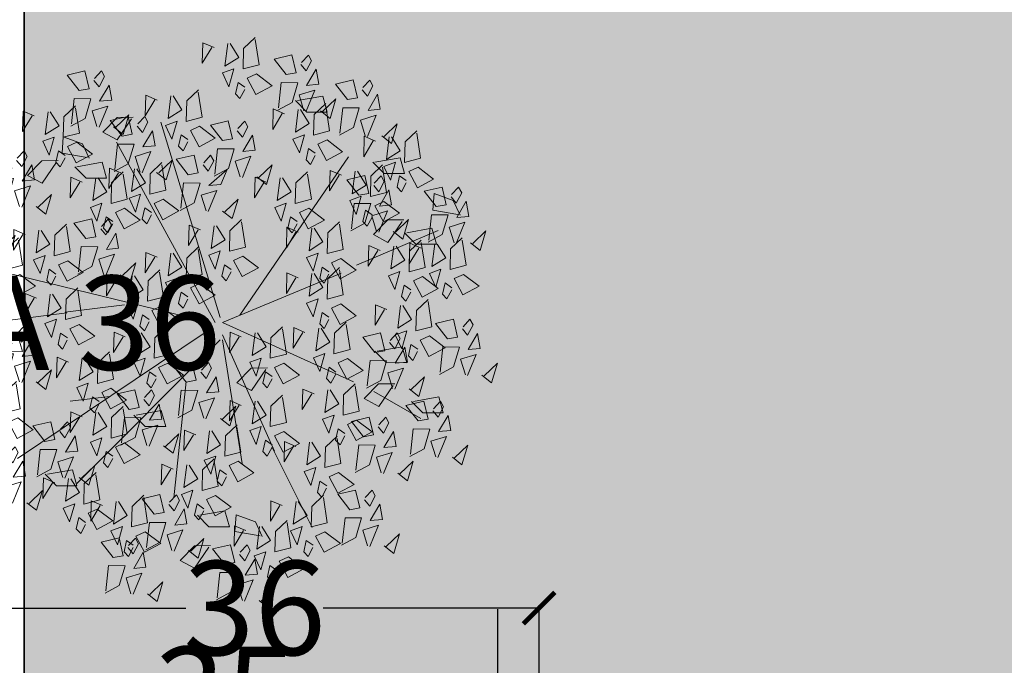
# Model space of a CAD drawing. Units: inches. Extents: x 1704 to 6393, y -157 to 1172.
# Tile 6 of 122: x 1898 to 1961, y 41 to 82. Entities that reach past the tile are written whole.
import ezdxf

# ---------------------------------------------------------------- set-up
doc = ezdxf.new("R2010")
doc.units = ezdxf.units.IN
doc.header["$MEASUREMENT"] = 0
for name, color, linetype, lineweight in [('A-ANNO-DIMS', 7, 'Continuous', 13), ('C-PROP', 7, 'Continuous', 35), ('L-shrub', 74, 'Continuous', 18)]:
    doc.layers.add(name, color=color, linetype=linetype, lineweight=lineweight)
doc.layers.add('L-PLNT-PATT', color=253, linetype='Continuous', lineweight=13, true_color=0x9abc8f)
doc.styles.get("Standard").update_dxf_attribs({"font": 'arial.ttf'})
doc.dimstyles.get("Standard").update_dxf_attribs({"dimtxt": 6, "dimasz": 2, "dimexe": 0.18, "dimexo": 0.0625, "dimgap": 0.09, "dimtad": 0, "dimtih": 1, "dimtoh": 1, "dimdec": 1, "dimzin": 0, "dimdsep": 46, "dimlunit": 3, "dimtxsty": 'Standard', "dimblk": 'ARCHTICK', "dimcen": 0.09, "dimadec": 0, "dimazin": 0, "dimtfac": 1, "dimtdec": 1, "dimtofl": 0, "dimtmove": 0, "dimatfit": 3, "dimfxl": 1, "dimtolj": 1, "dimtzin": 0, "dimarcsym": 0})

# ---------------------------------------------------------------- blocks, each defined once
blk = doc.blocks.new('flower shrub 3')
at = {"layer": 'L-shrub'}
for p, q in [((-130.41, 216.9), (-123.45, 236)), ((-123.45, 236), (-108.99, 242.75)), ((-109.76, 240.63), (-114.02, 215.74)), ((71.14, 221.55), (86.95, 226.01)), ((86.95, 226.01), (86.87, 205.67)), ((-114.02, 215.74), (-130.41, 216.9)), ((-96.02, 214.78), (-80.21, 219.24)), ((-80.21, 219.24), (-80.29, 198.91)), ((75.55, 196.68), (71.14, 221.55)), ((-91.61, 189.92), (-96.02, 214.78)), ((86.87, 205.67), (75.54, 194.43)), ((-80.29, 198.91), (-91.62, 187.66)), ((-166.05, 183.2), (-150.24, 187.65)), ((-150.24, 187.65), (-150.32, 167.32)), ((-104.33, 170.99), (-104.5, 186.95)), ((21.44, 185.45), (37.25, 189.91)), ((37.25, 189.91), (37.17, 169.58)), ((-161.64, 158.33), (-166.05, 183.2)), ((-102.88, 185.37), (-81.99, 171.19)), ((25.85, 160.59), (21.44, 185.45)), ((58.31, 161.96), (58.15, 177.93)), ((59.76, 176.34), (80.66, 162.16)), ((-150.32, 167.32), (-161.65, 156.07)), ((-89.82, 156.75), (-104.33, 170.99)), ((-81.99, 171.19), (-89.82, 156.75)), ((37.17, 169.58), (25.84, 158.33)), ((72.82, 147.73), (58.31, 161.96)), ((80.66, 162.16), (72.82, 147.73)), ((-227.04, 106.49), (-211.23, 110.94)), ((-211.23, 110.94), (-211.31, 90.61)), ((-222.63, 81.62), (-227.04, 106.49)), ((-211.31, 90.61), (-222.64, 79.36)), ((42.5, 35.62), (42.33, 51.58)), ((43.95, 50), (64.85, 35.82)), ((188.1, 20.61), (195.06, 39.71)), ((195.06, 39.71), (209.52, 46.47)), ((208.75, 44.35), (204.49, 19.45)), ((57.01, 21.38), (42.5, 35.62)), ((64.85, 35.82), (57.01, 21.38)), ((204.49, 19.45), (188.1, 20.61)), ((184.09, 9.47), (199.9, 13.93)), ((199.9, 13.93), (199.81, -6.4)), ((188.5, -15.39), (184.09, 9.47)), ((199.81, -6.4), (188.49, -17.65)), ((218.7, -20.78), (218.53, -4.82)), ((220.15, -6.4), (241.04, -20.58)), ((233.21, -35.02), (218.7, -20.78)), ((241.04, -20.58), (233.21, -35.02)), ((84.69, -53.7), (100.5, -49.25)), ((89.1, -78.57), (84.69, -53.7)), ((100.5, -49.25), (100.42, -69.58)), ((100.42, -69.58), (89.1, -80.83)), ((-205.99, -97.49), (-206.15, -81.53)), ((-204.54, -83.11), (-183.64, -97.29)), ((-191.47, -111.73), (-205.99, -97.49)), ((-183.64, -97.29), (-191.47, -111.73)), ((-161.53, -112.36), (-145.72, -107.91)), ((-157.12, -137.23), (-161.53, -112.36)), ((-145.72, -107.91), (-145.8, -128.24)), ((-179.93, -131.75), (-165.46, -125)), ((-186.88, -150.86), (-179.93, -131.75)), ((-166.23, -127.12), (-170.5, -152.01)), ((-145.8, -128.24), (-157.13, -139.49)), ((143.42, -141.69), (159.24, -137.24)), ((147.84, -166.56), (143.42, -141.69)), ((159.24, -137.24), (159.15, -157.57)), ((-170.5, -152.01), (-186.88, -150.86)), ((-163.07, -171.95), (-163.23, -155.98)), ((-161.62, -157.57), (-140.72, -171.75)), ((159.15, -157.57), (147.83, -168.82)), ((-148.55, -186.18), (-163.07, -171.95)), ((-140.72, -171.75), (-148.55, -186.18)), ((10.15, -195.84), (25.96, -191.38)), ((25.96, -191.38), (25.88, -211.71)), ((14.56, -220.7), (10.15, -195.84)), ((25.88, -211.71), (14.55, -222.96))]:
    blk.add_line(p, q, dxfattribs=at)
for points in [[(49.51, 264.41), (57.05, 273.94), (37.55, 279.71), (50.15, 266.57)], [(-81.5, 253.13), (-73.97, 262.66), (-93.47, 268.43), (-80.86, 255.29)], [(-50.38, 246.16), (-38.67, 261.64), (-30.06, 245.61), (-46.11, 237.01), (-50.38, 246.16)], [(3.73, 245.02), (9.98, 250.22), (-0.21, 255.59), (-5.82, 252.55), (1.56, 245.66)], [(24.26, 250.7), (23.13, 262.8), (8.21, 260.16), (24.26, 250.7)], [(49.36, 247.98), (33.81, 243.17), (28.98, 258.72), (50, 250.14)], [(-127.29, 233.74), (-121.04, 238.94), (-131.23, 244.31), (-136.84, 241.27), (-129.46, 234.38)], [(-106.76, 239.42), (-107.89, 251.52), (-122.81, 248.88), (-106.76, 239.42)], [(-81.65, 236.7), (-97.21, 231.89), (-102.03, 247.44), (-81.01, 238.86)], [(-84.31, 244.82), (-59.35, 248.66), (-55.26, 232.75), (-75.59, 233.29), (-86.57, 244.88)], [(130.84, 235.08), (138.37, 244.61), (118.87, 250.38), (131.48, 237.24)], [(-37.14, 234.51), (-41.84, 227.87), (-30.61, 225.31), (-25.97, 229.7), (-34.88, 234.45)], [(13.52, 230.35), (-1.79, 218.41), (-5.97, 236.12), (11.75, 240.29), (13.52, 230.35)], [(46.65, 222.9), (21.55, 225.63), (21.7, 242.05), (41.19, 236.28), (48.82, 222.26)], [(-117.5, 219.07), (-132.81, 207.13), (-136.99, 224.84), (-119.27, 229.01), (-117.5, 219.07)], [(-84.36, 211.62), (-109.47, 214.34), (-109.32, 230.77), (-89.83, 225), (-82.2, 210.98)], [(-80.47, 219.88), (-66.68, 228.54), (-58.01, 214.76), (-80.53, 217.63)], [(10.61, 212.31), (22.33, 227.8), (30.93, 211.77), (14.88, 203.17), (10.61, 212.31)], [(85.05, 215.69), (91.3, 220.89), (81.11, 226.26), (75.5, 223.22), (82.88, 216.33)], [(105.58, 221.37), (104.45, 233.47), (89.53, 230.83), (105.58, 221.37)], [(130.69, 218.65), (115.13, 213.84), (110.31, 229.39), (131.33, 220.81)], [(-156.55, 201.03), (-144.84, 216.52), (-136.23, 200.48), (-152.28, 191.89), (-156.55, 201.03)], [(-59.39, 140.01), (-93.72, 220.83)], [(-55.51, 223.72), (-51.3, 212.33), (-37.56, 218.73), (-55.51, 223.72)], [(-48.12, 205.55), (-36.41, 221.03), (-27.8, 205), (-43.85, 196.4), (-48.12, 205.55)], [(-82.06, 204.2), (-57.09, 208.04), (-53, 192.14), (-73.33, 192.68), (-84.31, 204.27)], [(-23.32, 210.97), (1.64, 214.81), (5.73, 198.9), (-14.6, 199.45), (-25.58, 211.03)], [(63.07, 192.21), (70.6, 201.74), (51.11, 207.51), (63.71, 194.37)], [(94.84, 201.02), (79.53, 189.08), (75.35, 206.79), (93.07, 210.96), (94.84, 201.02)], [(127.98, 193.57), (102.87, 196.3), (103.02, 212.72), (122.51, 206.95), (130.14, 192.93)], [(-190.49, 199.69), (-165.52, 203.53), (-161.43, 187.62), (-181.76, 188.17), (-192.74, 199.75)], [(-76.38, 203.98), (-81.2, 192.82), (-60.88, 192.27), (-76.44, 201.72)], [(23.85, 200.67), (19.16, 194.03), (30.38, 191.47), (35.02, 195.86), (26.11, 200.61)], [(65.66, 157.16), (92.63, 203.69)], [(146.65, 180.93), (154.18, 190.46), (134.69, 196.23), (147.29, 183.09)], [(-143.31, 189.39), (-148.01, 182.75), (-136.78, 180.19), (-132.14, 184.58), (-141.05, 189.33)], [(-92.8, 176.42), (-85.27, 185.95), (-104.76, 191.72), (-92.16, 178.58)], [(-78.21, 179.27), (-64.42, 187.93), (-55.75, 174.15), (-78.27, 177.02)], [(-34.88, 193.9), (-39.58, 187.26), (-28.35, 184.7), (-23.71, 189.09), (-32.62, 193.84)], [(-19.48, 186.04), (-5.68, 194.7), (2.98, 180.92), (-19.54, 183.79)], [(5.48, 189.88), (9.7, 178.48), (23.43, 184.88), (5.48, 189.88)], [(37.81, 178.51), (36.68, 190.61), (21.76, 187.96), (37.81, 178.51)], [(62.92, 175.78), (47.36, 170.98), (42.54, 186.52), (63.56, 177.95)], [(-187.68, 165.14), (-180.14, 174.67), (-199.64, 180.44), (-187.04, 167.3)], [(-186.64, 174.76), (-172.85, 183.42), (-164.18, 169.64), (-186.7, 172.51)], [(-161.68, 178.6), (-157.47, 167.2), (-143.73, 173.6), (-161.68, 178.6)], [(-122.67, 167.19), (-110.95, 182.67), (-102.35, 166.64), (-118.4, 158.05), (-122.67, 167.19)], [(-53.25, 183.11), (-49.04, 171.72), (-35.3, 178.12), (-53.25, 183.11)], [(17.28, 172.82), (23.53, 178.03), (13.34, 183.4), (7.73, 180.35), (15.12, 173.46)], [(121.39, 167.23), (120.26, 179.33), (105.34, 176.68), (121.39, 167.23)], [(218.93, 167.39), (226.47, 176.93), (206.97, 182.7), (219.58, 169.56)], [(-156.6, 165.85), (-131.64, 169.69), (-127.55, 153.78), (-147.87, 154.33), (-158.86, 165.91)], [(-138.59, 157.03), (-132.33, 162.23), (-142.52, 167.6), (-148.14, 164.56), (-140.75, 157.67)], [(-118.06, 162.71), (-119.19, 174.81), (-134.1, 172.17), (-118.06, 162.71)], [(-92.95, 159.99), (-108.51, 155.18), (-113.33, 170.73), (-92.31, 162.15)], [(-15.39, 170.13), (-20.21, 158.98), (0.12, 158.43), (-15.45, 167.88)], [(27.08, 158.16), (11.76, 146.22), (7.58, 163.93), (25.31, 168.09), (27.08, 158.16)], [(60.21, 150.7), (35.1, 153.43), (35.25, 169.85), (54.74, 164.09), (62.37, 150.06)], [(100.86, 161.54), (107.11, 166.75), (96.92, 172.11), (91.31, 169.07), (98.7, 162.18)], [(146.5, 164.5), (130.94, 159.7), (126.12, 175.24), (147.14, 166.67)], [(-233.46, 145.75), (-227.21, 150.95), (-237.4, 156.32), (-243.01, 153.28), (-235.63, 146.39)], [(-212.93, 151.43), (-214.06, 163.53), (-228.98, 160.89), (-212.93, 151.43)], [(-187.82, 148.71), (-203.38, 143.9), (-208.21, 159.45), (-187.18, 150.87)], [(-182.55, 158.85), (-187.37, 147.7), (-167.05, 147.15), (-182.61, 156.6)], [(-74.12, 163.36), (-78.94, 152.21), (-58.62, 151.66), (-74.18, 161.11)], [(110.66, 146.88), (95.35, 134.94), (91.16, 152.64), (108.89, 156.81), (110.66, 146.88)], [(143.79, 139.42), (118.68, 142.15), (118.83, 158.57), (138.33, 152.8), (145.96, 138.78)], [(173.15, 148), (179.4, 153.21), (169.21, 158.58), (163.6, 155.53), (170.98, 148.64)], [(193.68, 153.69), (192.55, 165.79), (177.63, 163.15), (193.68, 153.69)], [(218.79, 150.97), (203.23, 146.16), (198.41, 161.7), (219.43, 153.13)], [(-152.75, 140.92), (-138.96, 149.57), (-130.29, 135.8), (-152.82, 138.66)], [(-128.79, 142.36), (-144.1, 130.42), (-148.29, 148.13), (-130.56, 152.3), (-128.79, 142.36)], [(-95.66, 134.91), (-120.77, 137.64), (-120.62, 154.06), (-101.12, 148.29), (-93.49, 134.27)], [(-109.42, 155.55), (-114.12, 148.9), (-102.89, 146.34), (-98.26, 150.73), (-107.17, 155.49)], [(33.2, 131.09), (44.92, 146.57), (53.52, 130.54), (37.47, 121.95), (33.2, 131.09)], [(94.19, 140.12), (105.91, 155.6), (114.51, 139.57), (98.46, 130.97), (94.19, 140.12)], [(-223.67, 131.08), (-238.98, 119.14), (-243.16, 136.85), (-225.44, 141.02), (-223.67, 131.08)], [(-190.53, 123.63), (-215.64, 126.35), (-215.49, 142.78), (-196, 137.01), (-188.37, 122.99)], [(-127.79, 144.76), (-123.58, 133.36), (-109.85, 139.76), (-127.79, 144.76)], [(-66.19, 124.32), (-54.48, 139.81), (-45.87, 123.78), (-61.92, 115.18), (-66.19, 124.32)], [(-21.02, 124.32), (-9.3, 139.81), (-0.69, 123.78), (-16.74, 115.18), (-21.02, 124.32)], [(-2.54, 7.13), (56.31, 136.92)], [(60.26, 138.78), (85.22, 142.62), (89.31, 126.71), (68.99, 127.26), (58, 138.84)], [(146.15, 122.07), (157.86, 137.55), (166.47, 121.52), (150.42, 112.92), (146.15, 122.07)], [(182.94, 133.34), (167.63, 121.4), (163.45, 139.11), (181.17, 143.27), (182.94, 133.34)], [(216.08, 125.89), (190.97, 128.61), (191.12, 145.04), (210.61, 139.27), (218.24, 125.25)], [(-9.89, 24.27), (-166.82, 132.02)], [(-0.73, 129.75), (24.23, 133.59), (28.32, 117.68), (7.99, 118.23), (-2.99, 129.81)], [(107.43, 128.47), (102.74, 121.83), (113.97, 119.27), (118.6, 123.66), (109.69, 128.41)], [(-212.52, 104.22), (-204.99, 113.75), (-224.49, 119.52), (-211.88, 106.38)], [(-183.66, 110.79), (-171.94, 126.27), (-163.34, 110.24), (-179.39, 101.64), (-183.66, 110.79)], [(-148.66, 125.01), (-153.48, 113.86), (-133.16, 113.31), (-148.73, 122.75)], [(-100.13, 122.98), (-75.17, 126.82), (-71.08, 110.91), (-91.4, 111.46), (-102.39, 123.04)], [(-54.95, 122.98), (-29.99, 126.82), (-25.9, 110.91), (-46.22, 111.46), (-57.21, 123.04)], [(-2.54, 7.13), (-51.58, 124.68)], [(46.44, 119.45), (41.74, 112.81), (52.97, 110.25), (57.61, 114.63), (48.7, 119.39)], [(64.1, 113.85), (77.9, 122.5), (86.56, 108.73), (64.04, 111.59)], [(89.07, 117.69), (93.28, 106.29), (107.01, 112.69), (89.07, 117.69)], [(112.21, 120.73), (137.17, 124.57), (141.26, 108.66), (120.94, 109.21), (109.96, 120.79)], [(204.88, 108.53), (216.6, 124.01), (225.2, 107.98), (209.15, 99.39), (204.88, 108.53)], [(-217.59, 109.45), (-192.63, 113.29), (-188.54, 97.38), (-208.86, 97.93), (-219.85, 109.51)], [(-115.89, 92.74), (-104.17, 108.22), (-95.57, 92.19), (-111.62, 83.59), (-115.89, 92.74)], [(-52.95, 112.68), (-57.65, 106.04), (-46.42, 103.48), (-41.78, 107.87), (-50.69, 112.62)], [(-7.77, 112.68), (-12.47, 106.04), (-1.24, 103.48), (3.4, 107.87), (-5.51, 112.62)], [(3.11, 104.82), (16.91, 113.48), (25.57, 99.7), (3.05, 102.57)], [(28.07, 108.66), (32.29, 97.26), (46.02, 103.66), (28.07, 108.66)], [(159.39, 110.43), (154.69, 103.78), (165.92, 101.22), (170.56, 105.61), (161.65, 110.36)], [(170.95, 107.19), (195.91, 111.03), (200, 95.12), (179.67, 95.67), (168.69, 107.25)], [(-237.78, 90.52), (-238.91, 102.62), (-253.83, 99.97), (-237.78, 90.52)], [(-212.67, 87.79), (-228.23, 82.99), (-233.05, 98.53), (-212.03, 89.96)], [(-170.42, 99.14), (-175.11, 92.5), (-163.88, 89.94), (-159.25, 94.33), (-168.16, 99.08)], [(-96.28, 98.05), (-82.49, 106.71), (-73.82, 92.93), (-96.34, 95.8)], [(-71.32, 101.89), (-67.11, 90.49), (-53.38, 96.89), (-71.32, 101.89)], [(-51.1, 98.05), (-37.31, 106.71), (-28.64, 92.93), (-51.16, 95.8)], [(-26.14, 101.89), (-21.93, 90.49), (-8.2, 96.89), (-26.14, 101.89)], [(68.19, 97.94), (63.37, 86.78), (83.7, 86.23), (68.13, 95.68)], [(116.06, 95.8), (129.85, 104.45), (138.52, 90.68), (116, 93.54)], [(141.02, 99.64), (145.23, 88.24), (158.96, 94.64), (141.02, 99.64)], [(-258.31, 84.83), (-252.06, 90.04), (-262.25, 95.41), (-267.86, 92.36), (-260.48, 85.47)], [(-213.75, 84.52), (-199.95, 93.17), (-191.29, 79.4), (-213.81, 82.26)], [(-188.78, 88.36), (-184.57, 76.96), (-170.84, 83.36), (-188.78, 88.36)], [(-149.82, 91.4), (-124.86, 95.24), (-120.77, 79.33), (-141.1, 79.88), (-152.08, 91.46)], [(7.2, 88.91), (2.38, 77.76), (22.71, 77.21), (7.14, 86.66)], [(122.05, 56.75), (200.52, 95.93)], [(174.79, 82.26), (188.58, 90.91), (197.25, 77.14), (174.73, 80)], [(218.12, 96.89), (213.42, 90.24), (224.65, 87.68), (229.29, 92.07), (220.38, 96.83)], [(229.73, 72.43), (241.44, 87.91), (250.05, 71.88), (234, 63.29), (229.73, 72.43)], [(-248.51, 70.17), (-263.83, 58.23), (-268.01, 75.94), (-250.29, 80.1), (-248.51, 70.17)], [(-215.38, 62.71), (-240.49, 65.44), (-240.34, 81.86), (-220.85, 76.1), (-213.22, 62.07)], [(-102.65, 81.1), (-107.35, 74.45), (-96.12, 71.89), (-91.48, 76.28), (-100.39, 81.03)], [(-92.19, 82.14), (-97.01, 70.99), (-76.69, 70.44), (-92.25, 79.89)], [(-47.01, 82.14), (-51.83, 70.99), (-31.51, 70.44), (-47.07, 79.89)], [(37.72, 67.92), (49.43, 83.4), (58.04, 67.37), (41.99, 58.78), (37.72, 67.92)], [(105.49, 67.92), (117.2, 83.4), (125.81, 67.37), (109.76, 58.78), (105.49, 67.92)], [(120.15, 79.89), (115.33, 68.73), (135.65, 68.18), (120.09, 77.63)], [(199.75, 86.1), (203.97, 74.7), (217.7, 81.1), (199.75, 86.1)], [(-209.66, 68.61), (-214.48, 57.45), (-194.15, 56.9), (-209.72, 66.35)], [(-145.98, 66.47), (-132.19, 75.12), (-123.52, 61.35), (-146.04, 64.21)], [(-121.02, 70.31), (-116.8, 58.91), (-103.07, 65.31), (-121.02, 70.31)], [(3.78, 66.58), (28.75, 70.42), (32.84, 54.51), (12.51, 55.06), (1.53, 66.64)], [(71.55, 66.58), (96.51, 70.42), (100.6, 54.51), (80.28, 55.06), (69.29, 66.64)], [(195.79, 71.09), (220.76, 74.93), (224.85, 59.02), (204.52, 59.57), (193.54, 71.15)], [(178.88, 66.35), (174.06, 55.2), (194.39, 54.65), (178.82, 64.09)], [(242.97, 60.79), (238.27, 54.15), (249.5, 51.59), (254.14, 55.97), (245.23, 60.73)], [(273.15, 43.3), (280.68, 52.84), (261.19, 58.61), (273.79, 45.47)], [(-249.17, 40.85), (-237.45, 56.33), (-228.85, 40.3), (-244.9, 31.7), (-249.17, 40.85)], [(-147.01, 41.05), (-139.48, 50.58), (-158.98, 56.35), (-146.37, 43.21)], [(-141.89, 50.56), (-146.71, 39.4), (-126.38, 38.85), (-141.95, 48.3)], [(7.63, 41.65), (21.42, 50.3), (30.09, 36.53), (7.57, 39.39)], [(9.72, 7.13), (124.97, 58.56)], [(50.96, 56.28), (46.26, 49.63), (57.49, 47.07), (62.13, 51.46), (53.22, 56.22)], [(75.4, 41.65), (89.19, 50.3), (97.86, 36.53), (75.34, 39.39)], [(118.73, 56.28), (114.03, 49.63), (125.26, 47.07), (129.9, 51.46), (120.99, 56.22)], [(199.64, 46.16), (213.43, 54.82), (222.1, 41.04), (199.58, 43.91)], [(224.6, 50), (228.81, 38.6), (242.55, 45), (224.6, 50)], [(-283.1, 39.51), (-258.14, 43.35), (-254.05, 27.44), (-274.37, 27.98), (-285.36, 39.57)], [(-172.27, 27.35), (-173.4, 39.44), (-188.32, 36.8), (-172.27, 27.35)], [(-68.45, 27.31), (-56.74, 42.79), (-48.13, 26.76), (-64.18, 18.17), (-68.45, 27.31)], [(32.59, 45.49), (36.8, 34.09), (50.54, 40.49), (32.59, 45.49)], [(100.36, 45.49), (104.57, 34.09), (118.3, 40.49), (100.36, 45.49)], [(247.89, 29.6), (246.76, 41.7), (231.84, 39.06), (247.89, 29.6)], [(-192.8, 21.66), (-186.55, 26.86), (-196.74, 32.23), (-202.35, 29.19), (-194.97, 22.3)], [(-147.16, 24.62), (-162.72, 19.81), (-167.54, 35.36), (-146.52, 26.78)], [(-102.39, 25.97), (-77.43, 29.81), (-73.34, 13.9), (-93.66, 14.45), (-104.64, 26.03)], [(134.85, 22.8), (146.57, 38.28), (155.17, 22.25), (139.12, 13.65), (134.85, 22.8)], [(203.73, 30.25), (198.91, 19.1), (219.23, 18.55), (203.67, 28)], [(227.36, 23.91), (233.62, 29.12), (223.43, 34.49), (217.81, 31.44), (225.2, 24.55)], [(273, 26.88), (257.44, 22.07), (252.62, 37.61), (273.64, 29.04)], [(-279.26, 14.57), (-265.46, 23.23), (-256.8, 9.45), (-279.32, 12.32)], [(-235.92, 29.2), (-240.62, 22.56), (-229.39, 20), (-224.76, 24.39), (-233.67, 29.14)], [(-113.13, 7.2), (-105.6, 16.74), (-125.09, 22.51), (-112.49, 9.37)], [(11.72, 25.74), (6.9, 14.58), (27.22, 14.04), (11.66, 23.48)], [(14.63, 7.13), (137.23, 26.72)], [(79.49, 25.74), (74.67, 14.58), (94.99, 14.04), (79.43, 23.48)], [(92.43, 4.95), (99.97, 14.48), (80.47, 20.25), (93.07, 7.11)], [(100.92, 21.46), (125.88, 25.3), (129.97, 9.39), (109.65, 9.94), (98.66, 21.52)], [(270.29, 1.8), (245.18, 4.52), (245.33, 20.95), (264.83, 15.18), (272.46, 1.16)], [(-254.29, 18.41), (-250.08, 7.02), (-236.35, 13.42), (-254.29, 18.41)], [(-183.01, 6.99), (-198.32, -4.95), (-202.5, 12.76), (-184.78, 16.93), (-183.01, 6.99)], [(-149.87, -0.46), (-174.98, 2.27), (-174.83, 18.69), (-155.34, 12.92), (-147.71, -1.1)], [(-138.39, -6.5), (-139.52, 5.6), (-154.26, 11.88), (-138.39, -6.5)], [(-55.21, 15.67), (-59.91, 9.02), (-48.68, 6.46), (-44.04, 10.85), (-52.95, 15.61)], [(148.1, 11.15), (143.4, 4.51), (154.63, 1.95), (159.26, 6.34), (150.35, 11.09)], [(168.74, 0.24), (180.45, 15.72), (189.06, -0.31), (173.01, -8.91), (168.74, 0.24)], [(237.16, 9.25), (221.85, -2.69), (217.66, 15.02), (235.39, 19.19), (237.16, 9.25)], [(-7.44, 4.68), (-201.15, -54.09)], [(-113.28, -9.22), (-128.84, -14.03), (-133.66, 1.52), (-112.64, -7.06)], [(-98.54, 1.04), (-84.75, 9.69), (-76.08, -4.08), (-98.6, -1.22)], [(-73.58, 4.88), (-69.37, -6.52), (-55.64, -0.12), (-73.58, 4.88)], [(14.63, 4.68), (156.84, -137.36)], [(67.18, -8.75), (66.05, 3.35), (51.13, 0.7), (67.18, -8.75)], [(104.77, -3.47), (118.56, 5.18), (127.22, -8.59), (104.7, -5.73)], [(129.73, 0.37), (133.94, -11.03), (147.67, -4.63), (129.73, 0.37)], [(134.8, -1.11), (159.76, 2.73), (163.85, -13.17), (143.53, -12.63), (132.54, -1.04)], [(-275.17, -1.33), (-279.99, -12.49), (-259.66, -13.04), (-275.23, -3.59)], [(-197.21, -15.56), (-185.5, -0.08), (-176.89, -16.11), (-192.94, -24.7), (-197.21, -15.56)], [(-2.54, -0.22), (-181.53, -98.18)], [(-158.92, -12.19), (-152.66, -6.98), (-162.85, -1.61), (-168.47, -4.65), (-161.08, -11.54)], [(-2.54, -5.12), (-51.58, -205.93)], [(-41.35, -15.56), (-29.63, -0.08), (-21.02, -16.11), (-37.07, -24.7), (-41.35, -15.56)], [(46.65, -14.44), (52.9, -9.23), (42.71, -3.87), (37.1, -6.91), (44.48, -13.8)], [(92.28, -11.48), (76.73, -16.28), (71.9, -0.74), (92.92, -9.31)], [(-231.15, -16.9), (-206.18, -13.06), (-202.09, -28.97), (-222.42, -28.42), (-233.4, -16.84)], [(-149.12, -26.85), (-164.43, -38.79), (-168.62, -21.08), (-150.89, -16.91), (-149.12, -26.85)], [(-115.99, -34.3), (-141.1, -31.58), (-140.95, -15.15), (-121.45, -20.92), (-113.82, -34.94)], [(-94.45, -14.87), (-99.27, -26.03), (-78.95, -26.58), (-94.51, -17.13)], [(-75.28, -16.9), (-50.32, -13.06), (-46.23, -28.97), (-66.55, -28.42), (-77.54, -16.84)], [(7.27, -10.01), (132.32, -196.13)], [(56.44, -29.1), (41.13, -41.04), (36.95, -23.34), (54.67, -19.17), (56.44, -29.1)], [(89.57, -36.56), (64.47, -33.83), (64.62, -17.41), (84.11, -23.18), (91.74, -37.2)], [(108.86, -19.38), (104.03, -30.54), (124.36, -31.09), (108.79, -21.64)], [(138.65, -26.04), (152.44, -17.38), (161.11, -31.16), (138.59, -28.29)], [(181.98, -11.41), (177.28, -18.05), (188.51, -20.61), (193.15, -16.22), (184.24, -11.47)], [(223.45, -26.64), (230.99, -17.1), (211.49, -11.33), (224.09, -24.47)], [(-183.97, -27.2), (-188.67, -33.84), (-177.44, -36.4), (-172.8, -32.02), (-181.71, -27.26)], [(-28.1, -27.2), (-32.8, -33.84), (-21.57, -36.4), (-16.93, -32.02), (-25.84, -27.26)], [(55.85, -28.96), (171.09, -41.21)], [(163.61, -22.2), (167.82, -33.59), (181.55, -27.19), (163.61, -22.2)], [(198.2, -40.34), (197.06, -28.24), (182.15, -30.88), (198.2, -40.34)], [(-227.3, -41.83), (-213.51, -33.17), (-204.84, -46.95), (-227.36, -44.08)], [(-202.34, -37.99), (-198.13, -49.39), (-184.4, -42.99), (-202.34, -37.99)], [(-124.93, -51.66), (-113.21, -36.17), (-104.6, -52.2), (-120.65, -60.8), (-124.93, -51.66)], [(-71.43, -41.83), (-57.64, -33.17), (-48.97, -46.95), (-71.49, -44.08)], [(-46.47, -37.99), (-42.26, -49.39), (-28.53, -42.99), (-46.47, -37.99)], [(-18.76, -53.91), (-7.04, -38.43), (1.57, -54.46), (-14.48, -63.06), (-18.76, -53.91)], [(37.72, -47.14), (49.43, -31.66), (58.04, -47.69), (41.99, -56.29), (37.72, -47.14)], [(119.54, -51.46), (127.07, -41.92), (107.58, -36.15), (120.18, -49.29)], [(177.67, -46.03), (183.92, -40.82), (173.73, -35.45), (168.12, -38.5), (175.5, -45.39)], [(223.3, -43.06), (207.75, -47.87), (202.92, -32.33), (223.94, -40.9)], [(-151.53, -58.22), (-144, -48.69), (-163.49, -42.92), (-150.89, -56.06)], [(3.78, -48.48), (28.75, -44.64), (32.84, -60.55), (12.51, -60.01), (1.53, -48.42)], [(142.74, -41.95), (137.92, -53.1), (158.24, -53.65), (142.68, -44.2)], [(-223.21, -57.74), (-228.03, -68.89), (-207.71, -69.44), (-223.27, -59.99)], [(-158.86, -53), (-133.9, -49.16), (-129.81, -65.07), (-150.13, -64.52), (-161.12, -52.94)], [(-67.34, -57.74), (-72.16, -68.89), (-51.84, -69.44), (-67.4, -59.99)], [(-52.69, -55.25), (-27.73, -51.41), (-23.64, -67.32), (-43.96, -66.77), (-54.95, -55.19)], [(94.28, -65.16), (93.15, -53.06), (78.24, -55.7), (94.28, -65.16)], [(119.39, -67.88), (103.83, -72.69), (99.01, -57.14), (120.03, -65.72)], [(187.46, -60.69), (172.15, -72.63), (167.97, -54.92), (185.69, -50.76), (187.46, -60.69)], [(220.59, -68.14), (195.49, -65.42), (195.64, -48.99), (215.13, -54.76), (222.76, -68.78)], [(204.88, -69.71), (216.6, -54.22), (225.2, -70.25), (209.15, -78.85), (204.88, -69.71)], [(266.37, -67.25), (273.91, -57.71), (254.41, -51.94), (267.01, -65.08)], [(-197.32, -77.61), (-191.07, -72.41), (-201.26, -67.04), (-206.87, -70.08), (-199.48, -76.97)], [(-176.79, -71.93), (-177.92, -59.83), (-192.84, -62.47), (-176.79, -71.93)], [(-151.68, -74.65), (-167.24, -79.46), (-172.06, -63.91), (-151.04, -72.49)], [(-111.68, -63.3), (-116.38, -69.94), (-105.15, -72.5), (-100.51, -68.11), (-109.42, -63.36)], [(-5.51, -65.55), (-10.21, -72.2), (1.02, -74.76), (5.66, -70.37), (-3.25, -65.62)], [(7.63, -73.42), (21.42, -64.76), (30.09, -78.54), (7.57, -75.67)], [(50.96, -58.79), (46.26, -65.43), (57.49, -67.99), (62.13, -63.6), (53.22, -58.85)], [(73.75, -70.85), (80.01, -65.64), (69.82, -60.27), (64.2, -63.31), (71.59, -70.2)], [(170.95, -71.05), (195.91, -67.21), (200, -83.12), (179.67, -82.57), (168.69, -70.99)], [(-155.01, -77.93), (-141.22, -69.27), (-132.55, -83.05), (-155.07, -80.18)], [(-130.05, -74.09), (-125.84, -85.49), (-112.11, -79.09), (-130.05, -74.09)], [(-115.89, -90.01), (-104.17, -74.53), (-95.57, -90.56), (-111.62, -99.15), (-115.89, -90.01)], [(-48.84, -80.18), (-35.05, -71.53), (-26.38, -85.3), (-48.9, -82.44)], [(-23.88, -76.34), (-19.67, -87.74), (-5.94, -81.34), (-23.88, -76.34)], [(32.59, -69.58), (36.8, -80.97), (50.54, -74.57), (32.59, -69.58)], [(83.55, -85.51), (68.24, -97.45), (64.06, -79.74), (81.78, -75.57), (83.55, -85.51)], [(116.68, -92.96), (91.57, -90.24), (91.72, -73.81), (111.22, -79.58), (118.85, -93.6)], [(116.78, -90.01), (128.5, -74.53), (137.1, -90.56), (121.05, -99.15), (116.78, -90.01)], [(220.59, -86.64), (226.84, -81.43), (216.65, -76.06), (211.04, -79.11), (218.42, -86)], [(241.12, -80.95), (239.98, -68.85), (225.07, -71.49), (241.12, -80.95)], [(266.22, -83.67), (250.67, -88.48), (245.84, -72.94), (266.86, -81.51)], [(-196.71, -101.09), (-189.18, -91.56), (-208.67, -85.79), (-196.07, -98.93)], [(-187.52, -92.28), (-202.84, -104.22), (-207.02, -86.51), (-189.29, -82.34), (-187.52, -92.28)], [(-154.39, -99.73), (-179.5, -97), (-179.35, -80.58), (-159.85, -86.35), (-152.23, -100.37)], [(-149.82, -91.35), (-124.86, -87.51), (-120.77, -103.42), (-141.1, -102.87), (-152.08, -91.29)], [(-49.88, -94.32), (-42.35, -84.79), (-61.84, -79.02), (-49.24, -92.16)], [(82.85, -91.35), (107.81, -87.51), (111.9, -103.42), (91.58, -102.87), (80.59, -91.29)], [(174.79, -95.98), (188.58, -87.32), (197.25, -101.1), (174.73, -98.23)], [(218.12, -81.35), (213.42, -87.99), (224.65, -90.55), (229.29, -86.16), (220.38, -81.41)], [(-150.92, -93.84), (-155.74, -104.99), (-135.42, -105.54), (-150.98, -96.09)], [(-75.14, -108.02), (-76.27, -95.92), (-91.18, -98.57), (-75.14, -108.02)], [(-44.75, -96.09), (-49.57, -107.25), (-29.25, -107.8), (-44.81, -98.35)], [(-12.8, -148.96), (-20.16, -90.19)], [(11.72, -89.32), (6.9, -100.48), (27.22, -101.03), (11.66, -91.58)], [(62.57, -103.55), (74.28, -88.07), (82.89, -104.1), (66.84, -112.69), (62.57, -103.55)], [(199.75, -92.14), (203.97, -103.54), (217.7, -97.14), (199.75, -92.14)], [(230.38, -101.3), (215.07, -113.24), (210.89, -95.53), (228.61, -91.37), (230.38, -101.3)], [(263.51, -108.75), (238.41, -106.03), (238.56, -89.6), (258.05, -95.37), (265.68, -109.39)], [(-221.97, -114.79), (-223.1, -102.69), (-238.02, -105.34), (-221.97, -114.79)], [(-196.86, -117.52), (-212.42, -122.32), (-217.24, -106.78), (-196.22, -115.35)], [(-102.65, -101.65), (-107.35, -108.3), (-96.12, -110.86), (-91.48, -106.47), (-100.39, -101.71)], [(-95.67, -113.71), (-89.41, -108.5), (-99.6, -103.14), (-105.22, -106.18), (-97.83, -113.07)], [(-50.03, -110.75), (-65.59, -115.56), (-70.41, -100.01), (-49.39, -108.58)], [(28.63, -104.89), (53.59, -101.05), (57.68, -116.96), (37.36, -116.41), (26.37, -104.83)], [(70.56, -104.88), (75.47, -144.06)], [(130.02, -101.65), (125.33, -108.3), (136.56, -110.86), (141.19, -106.47), (132.28, -101.71)], [(182.29, -117.08), (194.01, -101.6), (202.61, -117.63), (186.56, -126.23), (182.29, -117.08)], [(-242.5, -120.48), (-236.24, -115.27), (-246.44, -109.9), (-252.05, -112.95), (-244.66, -119.84)], [(-145.98, -116.28), (-132.19, -107.63), (-123.52, -121.4), (-146.04, -118.54)], [(-121.02, -112.44), (-116.8, -123.84), (-103.07, -117.44), (-121.02, -112.44)], [(-52.74, -135.83), (-77.85, -133.1), (-77.7, -116.68), (-58.2, -122.45), (-50.57, -136.47)], [(75.81, -115.19), (71.11, -121.83), (82.34, -124.39), (86.98, -120.01), (78.07, -115.25)], [(86.69, -116.28), (100.49, -107.63), (109.15, -121.4), (86.63, -118.54)], [(111.65, -112.44), (115.87, -123.84), (129.6, -117.44), (111.65, -112.44)], [(148.36, -118.43), (173.32, -114.59), (177.41, -130.49), (157.08, -129.95), (146.1, -118.36)], [(178.88, -111.89), (174.06, -123.04), (194.39, -123.59), (178.82, -114.14)], [(-232.7, -135.14), (-248.01, -147.08), (-252.2, -129.38), (-234.47, -125.21), (-232.7, -135.14)], [(-199.57, -142.6), (-224.68, -139.87), (-224.53, -123.45), (-205.03, -129.21), (-197.4, -143.24)], [(-181.4, -137.39), (-169.68, -121.91), (-161.08, -137.94), (-177.13, -146.53), (-181.4, -137.39)], [(-85.87, -128.38), (-101.18, -140.31), (-105.37, -122.61), (-87.64, -118.44), (-85.87, -128.38)], [(-0.69, -135.13), (11.03, -119.65), (19.64, -135.68), (3.59, -144.28), (-0.69, -135.13)], [(32.48, -129.82), (46.27, -121.16), (54.94, -134.94), (32.42, -132.07)], [(57.44, -125.98), (61.65, -137.38), (75.38, -130.98), (57.44, -125.98)], [(151.17, -134.93), (158.7, -125.4), (139.2, -119.63), (151.81, -132.77)], [(-215.33, -138.73), (-190.37, -134.89), (-186.28, -150.8), (-206.61, -150.25), (-217.59, -138.67)], [(-141.89, -132.19), (-146.71, -143.35), (-126.38, -143.9), (-141.95, -134.45)], [(-63.94, -146.41), (-52.22, -130.93), (-43.61, -146.96), (-59.66, -155.56), (-63.94, -146.41)], [(-34.62, -136.47), (-9.66, -132.63), (-5.57, -148.54), (-25.89, -148), (-36.88, -136.41)], [(90.78, -132.19), (85.96, -143.35), (106.29, -143.9), (90.72, -134.45)], [(125.91, -148.63), (124.78, -136.54), (109.86, -139.18), (125.91, -148.63)], [(152.2, -143.36), (166, -134.7), (174.66, -148.48), (152.14, -145.61)], [(195.53, -128.73), (190.83, -135.37), (202.06, -137.93), (206.7, -133.54), (197.79, -128.79)], [(-97.87, -147.76), (-72.91, -143.92), (-68.82, -159.82), (-89.14, -159.28), (-100.13, -147.69)], [(36.57, -145.73), (31.75, -156.88), (52.07, -157.43), (36.51, -147.98)], [(105.38, -154.32), (111.63, -149.12), (101.44, -143.75), (95.83, -146.79), (103.21, -153.68)], [(151.02, -151.36), (135.46, -156.17), (130.64, -140.62), (151.66, -149.2)], [(177.16, -139.52), (181.38, -150.91), (195.11, -144.51), (177.16, -139.52)], [(-211.49, -163.66), (-197.69, -155.01), (-189.03, -168.78), (-211.55, -165.92)], [(-168.16, -149.03), (-172.86, -155.68), (-161.63, -158.24), (-156.99, -153.85), (-165.9, -149.09)], [(-30.77, -161.41), (-16.98, -152.75), (-8.31, -166.53), (-30.83, -163.66)], [(-12.34, -147.15), (-0.08, -242.66)], [(12.56, -146.78), (7.86, -153.42), (19.09, -155.98), (23.73, -151.59), (14.82, -146.84)], [(-186.53, -159.82), (-182.31, -171.22), (-168.58, -164.82), (-186.53, -159.82)], [(-117.65, -177.8), (-110.11, -168.26), (-129.61, -162.5), (-117.01, -175.64)], [(-94.02, -172.69), (-80.23, -164.03), (-71.56, -177.81), (-94.08, -174.94)], [(-50.69, -158.06), (-55.39, -164.7), (-44.16, -167.26), (-39.52, -162.87), (-48.43, -158.12)], [(-5.81, -157.57), (-1.6, -168.96), (12.13, -162.56), (-5.81, -157.57)], [(56.29, -177.8), (63.82, -168.26), (44.33, -162.5), (56.93, -175.64)], [(115.18, -168.99), (99.86, -180.93), (95.68, -163.22), (113.4, -159.05), (115.18, -168.99)], [(148.31, -176.44), (123.2, -173.71), (123.35, -157.29), (142.84, -163.06), (150.47, -177.08)], [(156.29, -159.27), (151.47, -170.42), (171.8, -170.97), (156.23, -161.52)], [(-69.06, -168.85), (-64.85, -180.24), (-51.12, -173.84), (-69.06, -168.85)], [(176.01, -186.82), (183.55, -177.29), (164.05, -171.52), (176.66, -184.66)], [(-207.4, -179.57), (-212.22, -190.73), (-191.89, -191.27), (-207.46, -181.83)], [(-142.9, -191.5), (-144.04, -179.4), (-158.95, -182.05), (-142.9, -191.5)], [(-117.8, -194.23), (-133.35, -199.03), (-138.18, -183.49), (-117.16, -192.06)], [(-50.38, -193.79), (-38.67, -178.31), (-30.06, -194.34), (-46.11, -202.94), (-50.38, -193.79)], [(-26.68, -177.31), (-31.5, -188.47), (-11.18, -189.02), (-26.74, -179.57)], [(31.03, -191.5), (29.9, -179.4), (14.99, -182.05), (31.03, -191.5)], [(56.14, -194.23), (40.58, -199.03), (35.76, -183.49), (56.78, -192.06)], [(91.93, -196.05), (103.65, -180.57), (112.25, -196.6), (96.2, -205.19), (91.93, -196.05)], [(-163.43, -197.19), (-157.18, -191.98), (-167.37, -186.61), (-172.98, -189.66), (-165.6, -196.55)], [(-89.93, -188.6), (-94.75, -199.75), (-74.43, -200.3), (-89.99, -190.85)], [(-84.31, -195.13), (-59.35, -191.29), (-55.26, -207.2), (-75.59, -206.66), (-86.57, -195.07)], [(10.5, -197.19), (16.76, -191.98), (6.57, -186.61), (0.95, -189.66), (8.34, -196.55)], [(58, -197.39), (82.96, -193.55), (87.05, -209.46), (66.73, -208.91), (55.74, -197.33)], [(150.76, -200.53), (149.63, -188.43), (134.71, -191.07), (150.76, -200.53)], [(175.87, -203.25), (160.31, -208.06), (155.49, -192.51), (176.51, -201.09)], [(-153.64, -211.85), (-168.95, -223.79), (-173.13, -206.08), (-155.41, -201.92), (-153.64, -211.85)], [(-120.51, -219.31), (-145.61, -216.58), (-145.47, -200.15), (-125.97, -205.92), (-118.34, -219.95)], [(-76.99, -213.9), (-69.45, -204.36), (-88.95, -198.59), (-76.35, -211.73)], [(20.3, -211.85), (4.99, -223.79), (0.8, -206.08), (18.53, -201.92), (20.3, -211.85)], [(53.43, -219.31), (28.32, -216.58), (28.47, -200.15), (47.97, -205.92), (55.6, -219.95)], [(130.23, -206.21), (136.48, -201.01), (126.29, -195.64), (120.68, -198.68), (128.06, -205.57)], [(-80.47, -220.07), (-66.68, -211.41), (-58.01, -225.19), (-80.53, -222.32)], [(-37.14, -205.44), (-41.84, -212.08), (-30.61, -214.64), (-25.97, -210.25), (-34.88, -205.5)], [(61.85, -222.32), (75.64, -213.67), (84.3, -227.44), (61.78, -224.58)], [(105.18, -207.69), (100.48, -214.34), (111.71, -216.9), (116.34, -212.51), (107.43, -207.75)], [(140.02, -220.88), (124.71, -232.82), (120.53, -215.11), (138.25, -210.94), (140.02, -220.88)], [(173.16, -228.33), (148.05, -225.61), (148.2, -209.18), (167.69, -214.95), (175.32, -228.97)], [(-122.77, -233.29), (-116.52, -228.08), (-126.71, -222.71), (-132.32, -225.76), (-124.94, -232.65)], [(-102.24, -227.6), (-103.37, -215.5), (-118.29, -218.14), (-102.24, -227.6)], [(-77.14, -230.32), (-92.69, -235.13), (-97.52, -219.59), (-76.5, -228.16)], [(-55.51, -216.23), (-51.3, -227.62), (-37.56, -221.22), (-55.51, -216.23)], [(86.81, -218.48), (91.02, -229.88), (104.75, -223.48), (86.81, -218.48)], [(-112.98, -247.95), (-128.29, -259.89), (-132.47, -242.18), (-114.75, -238.02), (-112.98, -247.95)], [(-79.85, -255.4), (-104.95, -252.68), (-104.8, -236.25), (-85.31, -242.02), (-77.68, -256.04)], [(-76.38, -235.97), (-81.2, -247.13), (-60.88, -247.68), (-76.44, -238.23)], [(65.94, -238.23), (61.11, -249.39), (81.44, -249.93), (65.87, -240.49)]]:
    blk.add_lwpolyline(points, dxfattribs=at)
blk = doc.blocks.new('_ArchTick')
at = {"color": 0, "linetype": 'ByBlock', "const_width": 0.15}
blk.add_lwpolyline([(-0.5, -0.5), (0.5, 0.5)], dxfattribs=at)
blk = doc.blocks.new('*D71')
at = {"layer": 'A-ANNO-DIMS', "color": 0, "lineweight": -2, "transparency": 16777216}
for p, q in [((1894.896, 38.988), (1894.896, 44.734)), ((1931.183, 38.988), (1931.183, 44.734)), ((1894.896, 44.554), (1908.656, 44.554)), ((1931.183, 44.554), (1917.422, 44.554))]:
    blk.add_line(p, q, dxfattribs=at)
at = {"layer": 'Defpoints', "color": 0, "lineweight": -3, "transparency": 16777216}
for p in [(1931.183, 44.554), (1894.896, 38.926), (1931.183, 38.926)]:
    blk.add_point(p, dxfattribs=at)
at = {"layer": 'A-ANNO-DIMS', "color": 0, "lineweight": -2, "transparency": 16777216, "xscale": 2, "yscale": 2, "zscale": 2, "rotation": 180}
blk.add_blockref('_ArchTick', (1894.896, 44.554), dxfattribs=at)
at = {"layer": 'A-ANNO-DIMS', "color": 0, "lineweight": -2, "transparency": 16777216, "xscale": 2, "yscale": 2, "zscale": 2}
blk.add_blockref('_ArchTick', (1931.183, 44.554), dxfattribs=at)
at = {"layer": 'A-ANNO-DIMS', "color": 0, "transparency": 16777216, "insert": (1913.039, 44.554), "char_height": 6, "attachment_point": 5}
blk.add_mtext('\\A1;36', dxfattribs=at)
blk = doc.blocks.new('*D86')
at = {"layer": 'A-ANNO-DIMS', "color": 0, "lineweight": -2, "transparency": 16777216}
for p, q in [((1893.767, 80.936), (1888.19, 80.936)), ((1888.37, 80.936), (1888.37, 65.933)), ((1888.37, 44.542), (1888.37, 59.544)), ((1893.767, 44.542), (1888.19, 44.542))]:
    blk.add_line(p, q, dxfattribs=at)
at = {"layer": 'Defpoints', "color": 0, "lineweight": -3, "transparency": 16777216}
for p in [(1893.829, 80.936), (1888.37, 44.542), (1893.829, 44.542)]:
    blk.add_point(p, dxfattribs=at)
at = {"layer": 'A-ANNO-DIMS', "color": 0, "lineweight": -2, "transparency": 16777216, "xscale": 2, "yscale": 2, "zscale": 2}
for p, rotation in [((1888.37, 80.936), 90), ((1888.37, 44.542), 270)]:
    blk.add_blockref('_ArchTick', p, dxfattribs=dict(at, rotation=rotation))
at = {"layer": 'A-ANNO-DIMS', "color": 0, "transparency": 16777216, "insert": (1888.37, 62.739), "char_height": 6, "attachment_point": 5}
blk.add_mtext('\\A1;SHRUB A 36', dxfattribs=at)
blk = doc.blocks.new('*D87')
at = {"layer": 'A-ANNO-DIMS', "color": 0, "lineweight": -2, "transparency": 16777216}
for p, q in [((1893.829, 44.479), (1893.829, 38.903)), ((1928.523, 44.479), (1928.523, 38.903)), ((1893.829, 39.083), (1906.768, 39.083)), ((1928.523, 39.083), (1915.584, 39.083))]:
    blk.add_line(p, q, dxfattribs=at)
at = {"layer": 'Defpoints', "color": 0, "lineweight": -3, "transparency": 16777216}
for p in [(1893.829, 44.542), (1928.523, 44.542), (1928.523, 39.083)]:
    blk.add_point(p, dxfattribs=at)
at = {"layer": 'A-ANNO-DIMS', "color": 0, "lineweight": -2, "transparency": 16777216, "xscale": 2, "yscale": 2, "zscale": 2, "rotation": 180}
blk.add_blockref('_ArchTick', (1893.829, 39.083), dxfattribs=at)
at = {"layer": 'A-ANNO-DIMS', "color": 0, "lineweight": -2, "transparency": 16777216, "xscale": 2, "yscale": 2, "zscale": 2}
blk.add_blockref('_ArchTick', (1928.523, 39.083), dxfattribs=at)
at = {"layer": 'A-ANNO-DIMS', "color": 0, "transparency": 16777216, "insert": (1911.176, 39.083), "char_height": 6, "attachment_point": 5}
blk.add_mtext('\\A1;35', dxfattribs=at)

msp = doc.modelspace()

# ---------------------------------------------------------------- hatches: boundary and pattern name
at = {"layer": 'L-PLNT-PATT', "transparency": 33554643}
h = msp.add_hatch(color=256, dxfattribs=at)
h.dxf.hatch_style = 1
h.paths.add_polyline_path([(1975.349, 202.213), (1898.349, 202.213), (1898.349, -3.787), (1975.349, -3.787)])

# ---------------------------------------------------------------- linework, layer by layer
at = {"layer": 'C-PROP'}
msp.add_line((1898.349, -3.787), (1898.349, 1033.213), dxfattribs=at)

# ---------------------------------------------------------------- block references
at = {"layer": 'L-shrub', "xscale": 0.0642956299502212, "yscale": 0.0642956299502212, "zscale": 0.0642956299502212, "rotation": 270}
msp.add_blockref('flower shrub 3', (1910.539, 62.588), dxfattribs=at)

# ---------------------------------------------------------------- dimensions: what is measured, and where the dimension line sits
at = {"layer": 'A-ANNO-DIMS'}
dim = msp.add_linear_dim(base=(1888.37, 44.542), p1=(1893.829, 80.936), p2=(1893.829, 44.542), angle=270, text='SHRUB A <>', dimstyle='Standard', override={"dimdec": 0, "dimlfac": 1, "dimrnd": 0, "dimzin": 0, "dimdsep": 46, "dimlunit": 2}, dxfattribs=at)
dim.commit()
dim.dimension.update_dxf_attribs({"geometry": '*D86', "text_midpoint": (1888.37, 62.739)})
for base, p1, p2, picture, middle in [((1931.183, 44.554), (1894.896, 38.926), (1931.183, 38.926), '*D71', (1913.039, 44.554)), ((1928.523, 39.083), (1893.829, 44.542), (1928.523, 44.542), '*D87', (1911.176, 39.083))]:
    dim = msp.add_linear_dim(base=base, p1=p1, p2=p2, dimstyle='Standard', override={"dimdec": 0, "dimlfac": 1, "dimrnd": 0, "dimzin": 0, "dimdsep": 46, "dimlunit": 2}, dxfattribs=at)
    dim.commit()
    dim.dimension.update_dxf_attribs({"geometry": picture, "text_midpoint": middle})

doc.saveas('drawing.dxf')
